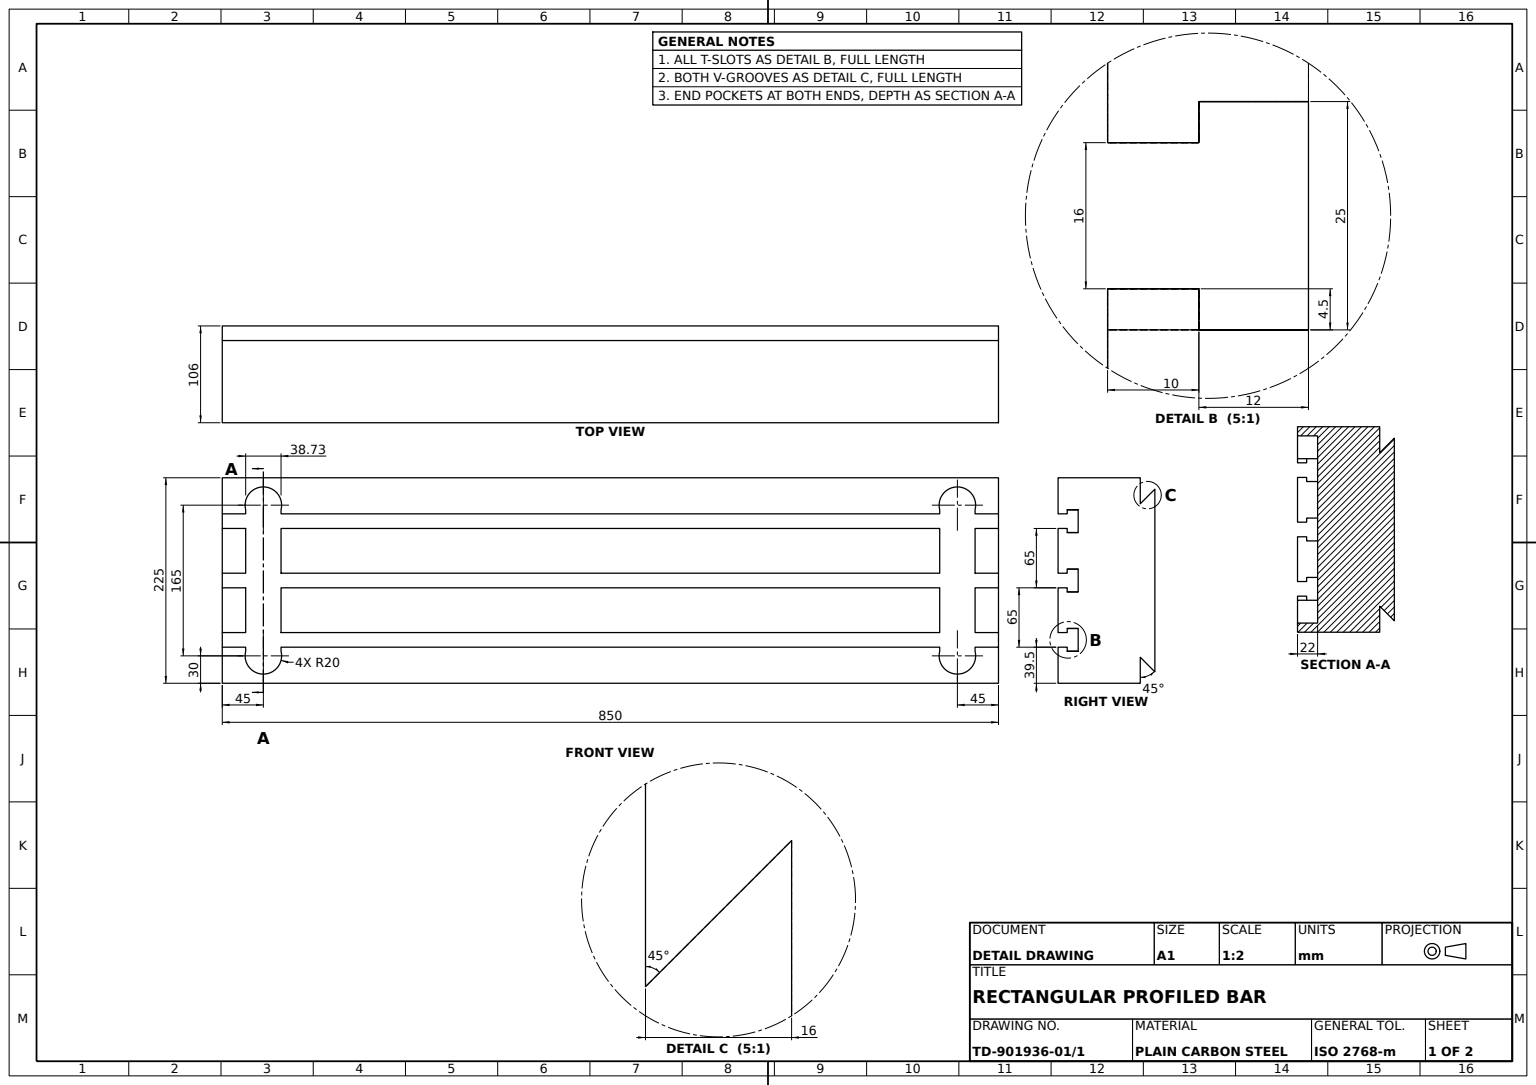
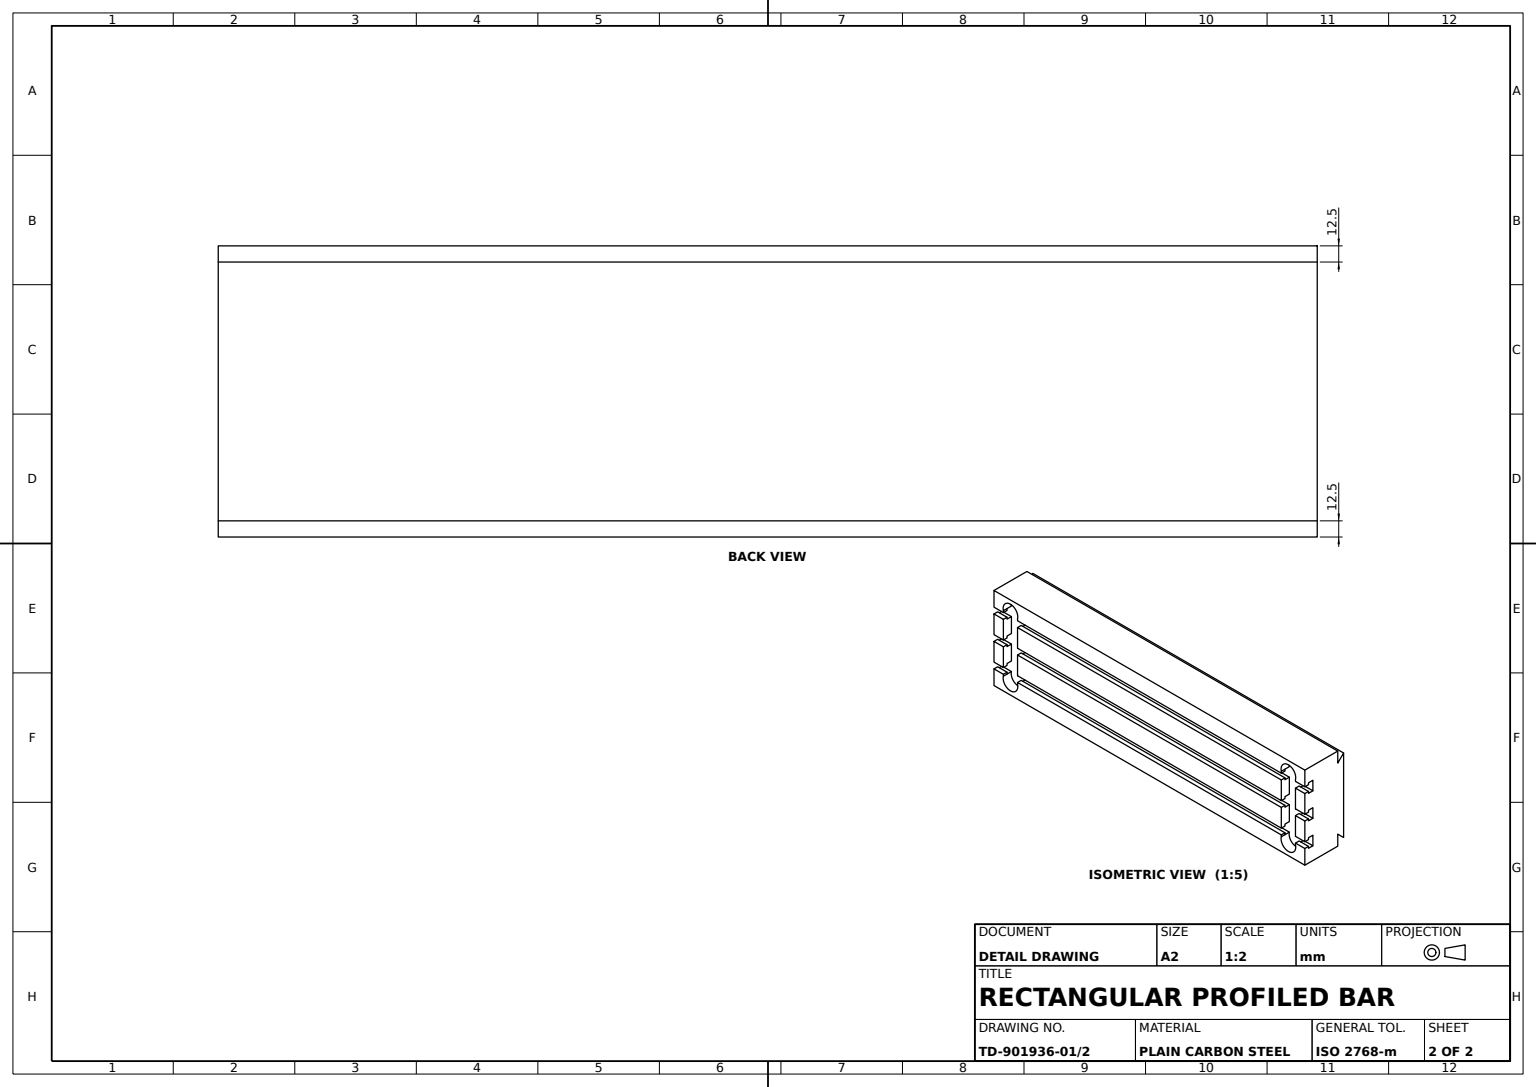
SolidWorks part; units mm, degrees
material "Plain Carbon Steel"
ref_plane "Front Plane" through (0, 0, 0) normal (0, 0, 1) x (1, 0, 0)
ref_plane "Top Plane" through (0, 0, 0) normal (0, 1, 0) x (1, 0, 0)
ref_plane "Right Plane" through (0, 0, 0) normal (1, 0, 0) x (0, 0, -1)
sketch "Base Block Profile" plane through (0, 0, 0) normal (0, 0, 1) x (1, 0, 0)
  line L1 (425, -112.5) -> (-425, -112.5)
  line L2 (425, -112.5) -> (425, 112.5)
  line L3 (425, 112.5) -> (-425, 112.5)
  line L4 (-425, -112.5) -> (-425, 112.5)
  line L5 (425, -112.5) -> (-425, 112.5) construction
  line L6 (425, 112.5) -> (-425, -112.5) construction
  point P0 (0, 0)
  dimension "D1" = 225
  dimension "D2" = 850
extrude "Base Block 850x225x106" add sketch "Base Block Profile" along normal blind 106
sketch "V-Groove Profile" plane through (425, 0, 0) normal (1, 0, 0) x (0, 0, -1)
  line L0 (-16, -112.5) -> (0, -112.5)
  line L2 (0, -112.5) -> (0, -100)
  line L3 (-106, -112.5) -> (0, -112.5) construction
  line L4 (0, -100) -> (-16, -84)
  line L5 (-16, -84) -> (-16, -112.5)
  line L6 (0, 0) -> (-261.6232, 0) construction
  line L7 (0, -112.5) -> (0, 112.5) construction
  line L8 (-16, 84) -> (-16, 112.5)
  line L9 (0, 100) -> (-16, 84)
  line L10 (0, 112.5) -> (0, 100)
  line L11 (-16, 112.5) -> (0, 112.5)
  point P6 (0, 0)
  dimension "D1" = 16
  dimension "D2" = 100
  dimension "D3" = 45
extrude "V-Groove 45deg" cut sketch "V-Groove Profile" against normal through all
sketch "T-Slots Profile" plane through (425, 0, 0) normal (1, 0, 0) x (0, 0, -1)
  line L0 (0, 0) -> (-214.294, 0) construction
  line L1 (-96, -12.5) -> (-84, -12.5)
  line L2 (-106, 8) -> (-96, 8)
  line L3 (-96, 8) -> (-96, 12.5)
  line L4 (-96, 12.5) -> (-84, 12.5)
  line L5 (-84, 12.5) -> (-84, -12.5)
  line L6 (-106, -112.5) -> (-106, 112.5) construction
  line L7 (-106, -8) -> (-106, 8)
  line L8 (-96, -8) -> (-96, -12.5)
  line L9 (-106, -8) -> (-96, -8)
  line L10 (0, 65) -> (-214.294, 65) construction
  line L11 (0, -65) -> (-214.294, -65) construction
  line L12 (-84, 77.5) -> (-84, 52.5)
  line L13 (-96, 73) -> (-96, 77.5)
  line L14 (-96, 57) -> (-96, 52.5)
  line L15 (-106, 57) -> (-106, 73)
  line L16 (-96, 52.5) -> (-84, 52.5)
  line L17 (-106, 73) -> (-96, 73)
  line L18 (-96, 77.5) -> (-84, 77.5)
  line L19 (-106, 57) -> (-96, 57)
  line L20 (-96, -77.5) -> (-84, -77.5)
  line L21 (-96, -57) -> (-96, -52.5)
  line L22 (-96, -73) -> (-96, -77.5)
  line L23 (-84, -52.5) -> (-84, -77.5)
  line L24 (-106, -73) -> (-106, -57)
  line L25 (-106, -57) -> (-96, -57)
  line L26 (-96, -52.5) -> (-84, -52.5)
  line L27 (-106, -73) -> (-96, -73)
  point P12 (-84, 0)
  point P24 (-85.147, 65)
  point P33 (-84, -65)
  dimension "D1" = 8
  dimension "D2" = 12.5
  dimension "D3" = 10
  dimension "D4" = 12
  dimension "D7" = 10
  dimension "D8" = 12
  dimension "D9" = 25
  dimension "D10" = 214.294
  dimension "D11" = 4.5
  dimension "D12" = 16
  dimension "D13" = 1.147
  dimension "D14" = 10
  dimension "D15" = 12
  dimension "D16" = 25
  dimension "D17" = 4.5
  dimension "D18" = 16
  dimension "D5" = 65
  dimension "D6" = 65
extrude "T-Slots 2x" cut sketch "T-Slots Profile" against normal through all
sketch "T-Slot End Pockets Profile" plane through (0, 0, 106) normal (0, 0, 1) x (1, 0, 0)
  line L0 (-425, 112.5) -> (-425, 73) construction
  line L1 (0, 0) -> (0, 272.3968) construction
  line L3 (-399.3632, -77.4932) -> (-399.3632, 77.4932)
  line L5 (-360.6368, -77.4932) -> (-360.6368, 77.4932)
  line L6 (360.6368, -77.4932) -> (360.6368, 77.4932)
  line L7 (399.3632, -77.4932) -> (399.3632, 77.4932)
  arc A0 (-360.6368, 77.4932) -> (-399.3632, 77.4932) centre (-380, 82.5) ccw
  arc A1 (-399.3632, -77.4932) -> (-360.6368, -77.4932) centre (-380, -82.5) ccw
  arc A2 (399.3632, -77.4932) -> (360.6368, -77.4932) centre (380, -82.5) cw
  arc A3 (360.6368, 77.4932) -> (399.3632, 77.4932) centre (380, 82.5) cw
  point P7 (-380, 0)
  point P18 (380, 0)
  dimension "D1" = 40
  dimension "D2" = 40
  dimension "D3" = 165
  dimension "D4" = 82.5
  dimension "D5" = 45
  dimension "D6" = 19.3632
  dimension "D7" = 19.3632
extrude "T-Slot End Pockets" cut sketch "T-Slot End Pockets Profile" against normal up to surface (22 mm away) up to face at (0, 0, 84)
